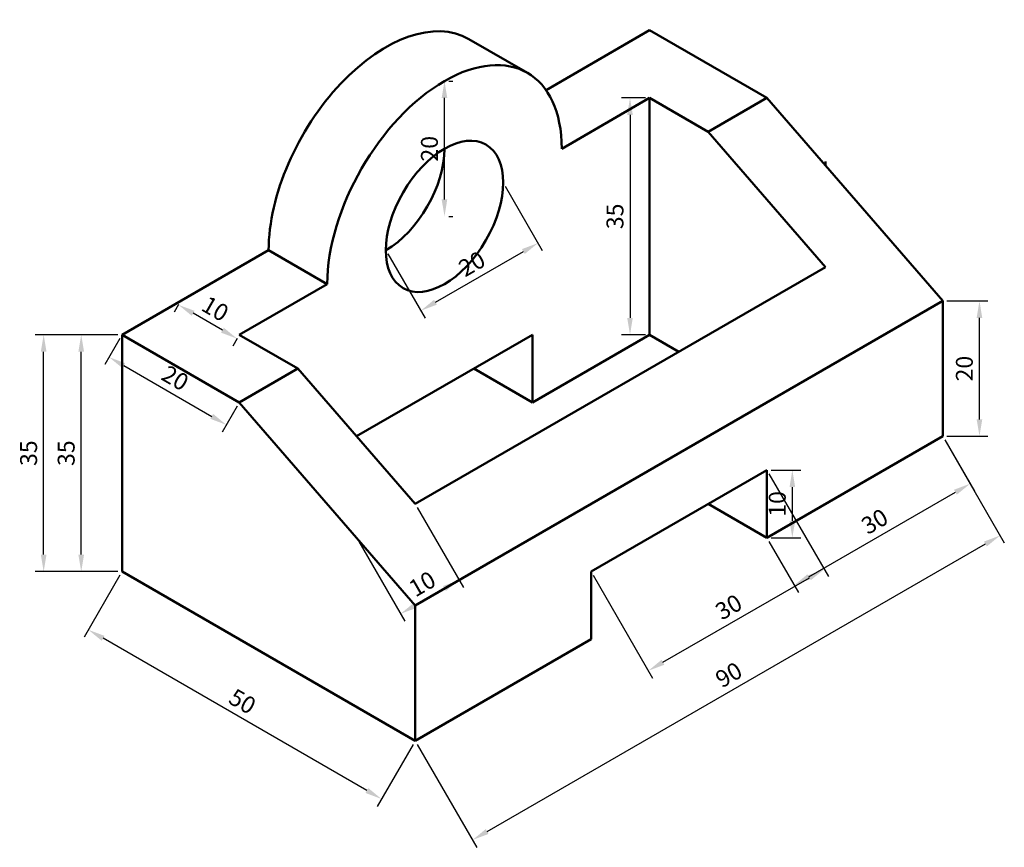
# Model space of a CAD drawing. Units: millimetres. Extents: x 93 to 239, y 58 to 180.
import ezdxf

# ---------------------------------------------------------------- set-up
doc = ezdxf.new("R2010")
doc.units = ezdxf.units.MM
doc.layers.add('M-DIMS', color=2, linetype='Continuous', lineweight=25)
doc.layers.add('M-OUTL', color=7, linetype='Continuous', lineweight=50)
doc.styles.get("Standard").update_dxf_attribs({"font": 'arial.ttf'})
doc.dimstyles.new('ISO-25', dxfattribs={"dimtxt": 2.5, "dimasz": 2.5, "dimexe": 1.25, "dimexo": 0.625, "dimtad": 1, "dimtxsty": 'Standard', "dimcen": 2.5, "dimadec": 0, "dimazin": 0, "dimtfac": 1, "dimtmove": 0, "dimatfit": 3, "dimfxl": 1, "dimarcsym": 0})

# ---------------------------------------------------------------- blocks, each defined once
blk = doc.blocks.new('*D1')
at = {"layer": 'Defpoints', "color": 0, "transparency": 16777216}
for p in [(203.57, 113.75), (212.03, 99.09), (177.59, 98.75)]:
    blk.add_point(p, dxfattribs=at)
at = {"layer": 'M-DIMS', "color": 0, "lineweight": -2, "transparency": 16777216}
for p, q in [((203.88, 113.21), (212.66, 98.01)), ((177.9, 98.21), (186.68, 83.01)), ((188.22, 85.34), (209.87, 97.84))]:
    blk.add_line(p, q, dxfattribs=at)
at = {"layer": 'M-DIMS', "color": 0, "transparency": 16777216}
for points in [[(209.66, 98.21), (210.07, 97.48), (212.03, 99.09)], [(188.01, 85.71), (188.42, 84.98), (186.05, 84.09)]]:
    blk.add_solid(points, dxfattribs=at)
at = {"layer": 'M-DIMS', "color": 0, "transparency": 16777216, "insert": (198.09, 93.24), "char_height": 2.5, "attachment_point": 5, "rotation": 30}
blk.add_mtext('30', dxfattribs=at)
blk = doc.blocks.new('*D2')
at = {"layer": 'Defpoints', "color": 0, "transparency": 16777216}
for p in [(229.55, 118.75), (233.6, 111.74), (203.57, 103.75)]:
    blk.add_point(p, dxfattribs=at)
at = {"layer": 'M-DIMS', "color": 0, "lineweight": -2, "transparency": 16777216}
for p, q in [((229.86, 118.21), (234.22, 110.66)), ((209.78, 97.99), (231.43, 110.49)), ((203.88, 103.21), (208.24, 95.66))]:
    blk.add_line(p, q, dxfattribs=at)
at = {"layer": 'M-DIMS', "color": 0, "transparency": 16777216}
for points in [[(231.22, 110.85), (231.64, 110.13), (233.6, 111.74)], [(209.57, 98.35), (209.99, 97.63), (207.62, 96.74)]]:
    blk.add_solid(points, dxfattribs=at)
at = {"layer": 'M-DIMS', "color": 0, "transparency": 16777216, "insert": (219.65, 105.89), "char_height": 2.5, "attachment_point": 5, "rotation": 30}
blk.add_mtext('30', dxfattribs=at)
blk = doc.blocks.new('*D3')
at = {"layer": 'Defpoints', "color": 0, "transparency": 16777216}
for p in [(229.55, 118.75), (238.02, 104.08), (151.61, 73.75)]:
    blk.add_point(p, dxfattribs=at)
at = {"layer": 'M-DIMS', "color": 0, "lineweight": -2, "transparency": 16777216}
for p, q in [((229.86, 118.21), (238.65, 102.99)), ((162.25, 60.33), (235.86, 102.83)), ((151.92, 73.21), (160.71, 57.99))]:
    blk.add_line(p, q, dxfattribs=at)
at = {"layer": 'M-DIMS', "color": 0, "transparency": 16777216}
for points in [[(235.65, 103.19), (236.07, 102.47), (238.02, 104.08)], [(162.04, 60.69), (162.45, 59.97), (160.08, 59.08)]]:
    blk.add_solid(points, dxfattribs=at)
at = {"layer": 'M-DIMS', "color": 0, "transparency": 16777216, "insert": (198.1, 83.22), "char_height": 2.5, "attachment_point": 5, "rotation": 30}
blk.add_mtext('90', dxfattribs=at)
blk = doc.blocks.new('*D4')
at = {"layer": 'Defpoints', "color": 0, "transparency": 16777216}
for p in [(108.31, 98.75), (103.33, 90.14), (151.61, 73.75)]:
    blk.add_point(p, dxfattribs=at)
at = {"layer": 'M-DIMS', "color": 0, "lineweight": -2, "transparency": 16777216}
for p, q in [((107.99, 98.21), (102.71, 89.05)), ((144.47, 66.39), (105.5, 88.89)), ((151.29, 73.21), (146.01, 64.05))]:
    blk.add_line(p, q, dxfattribs=at)
at = {"layer": 'M-DIMS', "color": 0, "transparency": 16777216}
for points in [[(105.71, 89.25), (105.29, 88.53), (103.33, 90.14)], [(144.68, 66.75), (144.26, 66.03), (146.63, 65.14)]]:
    blk.add_solid(points, dxfattribs=at)
at = {"layer": 'M-DIMS', "color": 0, "transparency": 16777216, "insert": (125.93, 79.28), "char_height": 2.5, "attachment_point": 5, "rotation": 330}
blk.add_mtext('50', dxfattribs=at)
blk = doc.blocks.new('*D5')
at = {"layer": 'Defpoints', "color": 0, "transparency": 16777216}
for p in [(102.27, 133.75), (108.31, 133.75), (108.31, 98.75)]:
    blk.add_point(p, dxfattribs=at)
at = {"layer": 'M-DIMS', "color": 0, "lineweight": -2, "transparency": 16777216}
for p, q in [((107.68, 133.75), (101.02, 133.75)), ((102.27, 101.25), (102.27, 131.25)), ((107.68, 98.75), (101.02, 98.75))]:
    blk.add_line(p, q, dxfattribs=at)
at = {"layer": 'M-DIMS', "color": 0, "transparency": 16777216}
for points in [[(101.85, 131.25), (102.69, 131.25), (102.27, 133.75)], [(101.85, 101.25), (102.69, 101.25), (102.27, 98.75)]]:
    blk.add_solid(points, dxfattribs=at)
at = {"layer": 'M-DIMS', "color": 0, "transparency": 16777216, "insert": (100.37, 116.25), "char_height": 2.5, "attachment_point": 5, "rotation": 90}
blk.add_mtext('35', dxfattribs=at)
blk = doc.blocks.new('*D6')
at = {"layer": 'Defpoints', "color": 0, "transparency": 16777216}
for p in [(164.6, 156.25), (169.76, 147.31), (147.28, 146.25)]:
    blk.add_point(p, dxfattribs=at)
at = {"layer": 'M-DIMS', "color": 0, "lineweight": -2, "transparency": 16777216}
for p, q in [((164.91, 155.71), (170.38, 146.23)), ((147.59, 145.71), (153.06, 136.23)), ((154.6, 138.56), (167.59, 146.06))]:
    blk.add_line(p, q, dxfattribs=at)
at = {"layer": 'M-DIMS', "color": 0, "transparency": 16777216}
for points in [[(167.39, 146.42), (167.8, 145.7), (169.76, 147.31)], [(154.4, 138.92), (154.81, 138.2), (152.44, 137.31)]]:
    blk.add_solid(points, dxfattribs=at)
at = {"layer": 'M-DIMS', "color": 0, "transparency": 16777216, "insert": (160.15, 143.96), "char_height": 2.5, "attachment_point": 5, "rotation": 30}
blk.add_mtext('20', dxfattribs=at)
blk = doc.blocks.new('*D7')
at = {"layer": 'Defpoints', "color": 0, "transparency": 16777216}
for p in [(155.94, 171.25), (155.94, 171.25), (155.94, 151.25)]:
    blk.add_point(p, dxfattribs=at)
at = {"layer": 'M-DIMS', "color": 0, "lineweight": -2, "transparency": 16777216}
for p, q in [((156.56, 171.25), (157.19, 171.25)), ((155.94, 153.75), (155.94, 168.75)), ((156.56, 151.25), (157.19, 151.25))]:
    blk.add_line(p, q, dxfattribs=at)
at = {"layer": 'M-DIMS', "color": 0, "transparency": 16777216}
for points in [[(155.52, 168.75), (156.35, 168.75), (155.94, 171.25)], [(155.52, 153.75), (156.35, 153.75), (155.94, 151.25)]]:
    blk.add_solid(points, dxfattribs=at)
at = {"layer": 'M-DIMS', "color": 0, "transparency": 16777216, "insert": (154.04, 161.25), "char_height": 2.5, "attachment_point": 5, "rotation": 90}
blk.add_mtext('20', dxfattribs=at)
blk = doc.blocks.new('*D8')
at = {"layer": 'Defpoints', "color": 0, "transparency": 16777216}
for p in [(116.97, 138.75), (116.63, 138.18), (125.63, 133.75)]:
    blk.add_point(p, dxfattribs=at)
at = {"layer": 'M-DIMS', "color": 0, "lineweight": -2, "transparency": 16777216}
for p, q in [((116.65, 138.21), (116.01, 137.09)), ((123.13, 134.43), (118.8, 136.93)), ((125.31, 133.21), (124.67, 132.09))]:
    blk.add_line(p, q, dxfattribs=at)
at = {"layer": 'M-DIMS', "color": 0, "transparency": 16777216}
for points in [[(119.01, 137.29), (118.59, 136.57), (116.63, 138.18)], [(123.34, 134.79), (122.92, 134.07), (125.29, 133.18)]]:
    blk.add_solid(points, dxfattribs=at)
at = {"layer": 'M-DIMS', "color": 0, "transparency": 16777216, "insert": (121.91, 137.32), "char_height": 2.5, "attachment_point": 5, "rotation": 330}
blk.add_mtext('10', dxfattribs=at)
blk = doc.blocks.new('*D9')
at = {"layer": 'Defpoints', "color": 0, "transparency": 16777216}
for p in [(186.25, 168.75), (183.35, 133.75), (186.25, 133.75)]:
    blk.add_point(p, dxfattribs=at)
at = {"layer": 'M-DIMS', "color": 0, "lineweight": -2, "transparency": 16777216}
for p, q in [((185.62, 168.75), (182.1, 168.75)), ((183.35, 166.25), (183.35, 136.25)), ((185.62, 133.75), (182.1, 133.75))]:
    blk.add_line(p, q, dxfattribs=at)
at = {"layer": 'M-DIMS', "color": 0, "transparency": 16777216}
for points in [[(182.93, 166.25), (183.76, 166.25), (183.35, 168.75)], [(182.93, 136.25), (183.76, 136.25), (183.35, 133.75)]]:
    blk.add_solid(points, dxfattribs=at)
at = {"layer": 'M-DIMS', "color": 0, "transparency": 16777216, "insert": (181.45, 151.25), "char_height": 2.5, "attachment_point": 5, "rotation": 90}
blk.add_mtext('35', dxfattribs=at)
blk = doc.blocks.new('*D10')
at = {"layer": 'Defpoints', "color": 0, "transparency": 16777216}
for p in [(151.61, 108.75), (142.95, 103.75), (149.44, 92.5)]:
    blk.add_point(p, dxfattribs=at)
at = {"layer": 'M-DIMS', "color": 0, "lineweight": -2, "transparency": 16777216}
for p, q in [((151.92, 108.21), (158.73, 96.42)), ((143.26, 103.21), (150.07, 91.42)), ((155.94, 96.25), (151.61, 93.75))]:
    blk.add_line(p, q, dxfattribs=at)
at = {"layer": 'M-DIMS', "color": 0, "transparency": 16777216}
for points in [[(155.73, 96.61), (156.15, 95.89), (158.1, 97.5)], [(151.4, 94.11), (151.82, 93.39), (149.44, 92.5)]]:
    blk.add_solid(points, dxfattribs=at)
at = {"layer": 'M-DIMS', "color": 0, "transparency": 16777216, "insert": (152.82, 96.65), "char_height": 2.5, "attachment_point": 5, "rotation": 30}
blk.add_mtext('10', dxfattribs=at)
blk = doc.blocks.new('*D11')
at = {"layer": 'Defpoints', "color": 0, "transparency": 16777216}
for p in [(229.55, 138.75), (234.98, 138.75), (229.55, 118.75)]:
    blk.add_point(p, dxfattribs=at)
at = {"layer": 'M-DIMS', "color": 0, "lineweight": -2, "transparency": 16777216}
for p, q in [((230.17, 138.75), (236.23, 138.75)), ((234.98, 121.25), (234.98, 136.25)), ((230.17, 118.75), (236.23, 118.75))]:
    blk.add_line(p, q, dxfattribs=at)
at = {"layer": 'M-DIMS', "color": 0, "transparency": 16777216}
for points in [[(234.56, 136.25), (235.39, 136.25), (234.98, 138.75)], [(234.56, 121.25), (235.39, 121.25), (234.98, 118.75)]]:
    blk.add_solid(points, dxfattribs=at)
at = {"layer": 'M-DIMS', "color": 0, "transparency": 16777216, "insert": (233.07, 128.75), "char_height": 2.5, "attachment_point": 5, "rotation": 90}
blk.add_mtext('20', dxfattribs=at)
blk = doc.blocks.new('*D12')
at = {"layer": 'Defpoints', "color": 0, "transparency": 16777216}
for p in [(108.31, 133.75), (125.63, 123.75), (123.71, 120.44)]:
    blk.add_point(p, dxfattribs=at)
at = {"layer": 'M-DIMS', "color": 0, "lineweight": -2, "transparency": 16777216}
for p, q in [((107.99, 133.21), (105.77, 129.35)), ((108.56, 129.19), (121.55, 121.69)), ((125.31, 123.21), (123.09, 119.35))]:
    blk.add_line(p, q, dxfattribs=at)
at = {"layer": 'M-DIMS', "color": 0, "transparency": 16777216}
for points in [[(108.76, 129.55), (108.35, 128.83), (106.39, 130.44)], [(121.76, 122.05), (121.34, 121.33), (123.71, 120.44)]]:
    blk.add_solid(points, dxfattribs=at)
at = {"layer": 'M-DIMS', "color": 0, "transparency": 16777216, "insert": (116, 127.08), "char_height": 2.5, "attachment_point": 5, "rotation": 330}
blk.add_mtext('20', dxfattribs=at)
blk = doc.blocks.new('*D13')
at = {"layer": 'Defpoints', "color": 0, "transparency": 16777216}
for p in [(203.57, 113.75), (203.57, 103.75), (207.33, 103.75)]:
    blk.add_point(p, dxfattribs=at)
at = {"layer": 'M-DIMS', "color": 0, "lineweight": -2, "transparency": 16777216}
for p, q in [((204.19, 113.75), (208.58, 113.75)), ((207.33, 111.25), (207.33, 106.25)), ((204.19, 103.75), (208.58, 103.75))]:
    blk.add_line(p, q, dxfattribs=at)
at = {"layer": 'M-DIMS', "color": 0, "transparency": 16777216}
for points in [[(206.92, 111.25), (207.75, 111.25), (207.33, 113.75)], [(206.92, 106.25), (207.75, 106.25), (207.33, 103.75)]]:
    blk.add_solid(points, dxfattribs=at)
at = {"layer": 'M-DIMS', "color": 0, "transparency": 16777216, "insert": (205.43, 108.75), "char_height": 2.5, "attachment_point": 5, "rotation": 90}
blk.add_mtext('10', dxfattribs=at)
blk = doc.blocks.new('*D14')
at = {"layer": 'Defpoints', "color": 0, "transparency": 16777216}
for p in [(96.72, 133.75), (108.31, 133.75), (108.31, 98.75)]:
    blk.add_point(p, dxfattribs=at)
at = {"layer": 'M-DIMS', "color": 0, "lineweight": -2, "transparency": 16777216}
for p, q in [((107.68, 133.75), (95.47, 133.75)), ((96.72, 101.25), (96.72, 131.25)), ((107.68, 98.75), (95.47, 98.75))]:
    blk.add_line(p, q, dxfattribs=at)
at = {"layer": 'M-DIMS', "color": 0, "transparency": 16777216}
for points in [[(96.3, 131.25), (97.14, 131.25), (96.72, 133.75)], [(96.3, 101.25), (97.14, 101.25), (96.72, 98.75)]]:
    blk.add_solid(points, dxfattribs=at)
at = {"layer": 'M-DIMS', "color": 0, "transparency": 16777216, "insert": (94.82, 116.25), "char_height": 2.5, "attachment_point": 5, "rotation": 90}
blk.add_mtext('35', dxfattribs=at)

msp = doc.modelspace()

# ---------------------------------------------------------------- linework, layer by layer
at = {"layer": 'M-OUTL'}
for p, q in [((170.937, 169.912), (186.248, 178.752)), ((186.248, 178.752), (203.569, 168.752)), ((168.185, 172.465), (159.524, 177.465)), ((173.258, 161.252), (186.248, 168.752)), ((186.248, 168.752), (194.908, 163.752)), ((186.248, 168.752), (186.248, 133.752)), ((186.248, 168.752), (194.908, 163.752)), ((194.908, 163.752), (203.569, 168.752)), ((203.569, 168.752), (229.549, 138.752)), ((194.908, 163.752), (212.229, 143.752)), ((212.229, 159.37), (212.229, 158.752)), ((108.306, 133.752), (129.956, 146.252)), ((138.617, 141.252), (129.956, 146.252)), ((151.607, 108.752), (212.229, 143.752)), ((125.626, 133.752), (138.617, 141.252)), ((229.549, 138.752), (151.607, 93.752)), ((229.549, 118.752), (229.549, 138.752)), ((108.306, 98.752), (108.306, 133.752)), ((108.306, 133.752), (125.626, 123.752)), ((134.287, 128.752), (125.626, 133.752)), ((142.947, 118.752), (168.928, 133.752)), ((168.928, 133.752), (168.928, 123.752)), ((168.928, 123.752), (186.248, 133.752)), ((186.248, 133.752), (190.578, 131.252)), ((125.626, 123.752), (134.287, 128.752)), ((134.287, 128.752), (151.607, 108.752)), ((168.928, 123.752), (160.267, 128.752)), ((151.607, 93.752), (125.626, 123.752)), ((203.569, 103.752), (229.549, 118.752)), ((177.588, 98.752), (203.569, 113.752)), ((203.569, 113.752), (203.569, 103.752)), ((194.908, 108.752), (203.569, 103.752)), ((151.607, 73.752), (108.306, 98.752)), ((177.588, 88.752), (177.588, 98.752)), ((151.607, 93.752), (151.607, 73.752)), ((151.607, 73.752), (177.588, 88.752))]:
    msp.add_line(p, q, dxfattribs=at)
for centre, major_axis, start_param in [((147.277, 156.252), (-12.247, -21.213), 3.1415927), ((155.937, 151.252), (-12.247, -21.213), 2.3561945), ((147.277, 156.252), (6.124, 10.607), 3.9269908)]:
    msp.add_ellipse(centre, major_axis=major_axis, ratio=0.5773503, start_param=start_param, end_param=5.4977871, dxfattribs=at)
msp.add_ellipse((155.937, 151.252), major_axis=(-6.124, -10.607), ratio=0.5773503, dxfattribs=at)

# ---------------------------------------------------------------- dimensions: what is measured, and where the dimension line sits
at = {"layer": 'M-DIMS'}
for base, p1, p2, override, picture, middle in [((155.937, 171.252), (155.937, 151.252), (155.937, 171.252), {"dimclrd": 0, "dimclre": 0, "dimclrt": 0}, '*D7', (154.036, 161.252)), ((183.348, 133.752), (186.248, 168.752), (186.248, 133.752), {"dimclrd": 0, "dimclre": 0, "dimclrt": 0}, '*D9', (181.446, 151.252)), ((234.976, 138.752), (229.549, 118.752), (229.549, 138.752), {"dimclrd": 0, "dimclre": 0, "dimclrt": 0}, '*D11', (233.074, 128.752)), ((96.721, 133.752), (108.306, 98.752), (108.306, 133.752), {"dimrnd": 0}, '*D14', (94.819, 116.252)), ((102.27, 133.752), (108.306, 98.752), (108.306, 133.752), {"dimclrd": 0, "dimclre": 0, "dimclrt": 0}, '*D5', (100.368, 116.252)), ((207.333, 103.752), (203.569, 113.752), (203.569, 103.752), {"dimclrd": 0, "dimclre": 0, "dimclrt": 0}, '*D13', (205.432, 108.752))]:
    dim = msp.add_linear_dim(base=base, p1=p1, p2=p2, angle=90, dimstyle='ISO-25', override=override, dxfattribs=at)
    dim.commit()
    dim.dimension.update_dxf_attribs({"geometry": picture, "text_midpoint": middle})
for p1, p2, distance, picture, middle in [((147.277, 146.252), (164.597, 156.252), -10.324, '*D6', (160.148, 143.958)), ((125.626, 133.752), (116.966, 138.752), 0.664, '*D8', (121.915, 137.323)), ((108.306, 133.752), (125.626, 123.752), -3.829, '*D12', (116.002, 127.083)), ((151.607, 73.752), (229.549, 118.752), -16.947, '*D3', (198.101, 83.223)), ((203.569, 103.752), (229.549, 118.752), -8.094, '*D2', (219.655, 105.89)), ((177.588, 98.752), (203.569, 113.752), -16.925, '*D1', (198.09, 93.242)), ((151.607, 108.752), (142.947, 103.752), 12.99, '*D10', (152.821, 96.649)), ((151.607, 73.752), (108.306, 98.752), 9.948, '*D4', (125.933, 79.283))]:
    dim = msp.add_aligned_dim(p1=p1, p2=p2, distance=distance, dimstyle='ISO-25', override={"dimclrd": 0, "dimclre": 0, "dimclrt": 0}, dxfattribs=at)
    dim.commit()
    dim.dimension.update_dxf_attribs({"geometry": picture, "text_midpoint": middle})

doc.saveas('drawing.dxf')
